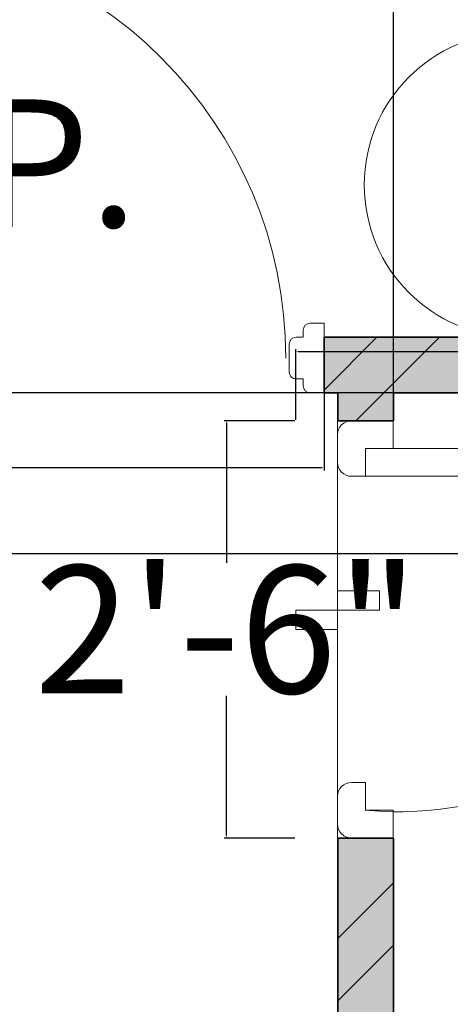
# Model space of a CAD drawing. Units: inches. Extents: x 1086 to 1540, y 3343 to 3848.
# Tile 4 of 8: x 1350 to 1381, y 3591 to 3661. Entities that reach past the tile are written whole.
import ezdxf

# ---------------------------------------------------------------- set-up
doc = ezdxf.new("R2010")
doc.units = ezdxf.units.IN
for name, color, linetype, lineweight in [('00 FURNITURE', 15, 'Continuous', 15), ('A-ANNO-DIMS', 2, 'Continuous', 13), ('A-DOOR', 4, 'Continuous', 20), ('A-WALL-PATT', 252, 'Continuous', 9), ('A_FUR 1', 5, 'Continuous', 5), ('WALL', 7, 'Continuous', 35)]:
    doc.layers.add(name, color=color, linetype=linetype, lineweight=lineweight)
doc.styles.get("Standard").update_dxf_attribs({"font": 'arial.ttf'})
doc.dimstyles.get("Standard").update_dxf_attribs({"dimtxt": 9.18, "dimasz": 0.18, "dimexe": 0.18, "dimexo": 0.0625, "dimgap": 0.09, "dimtad": 0, "dimtih": 1, "dimtoh": 1, "dimdec": 1, "dimzin": 0, "dimdsep": 46, "dimlunit": 3, "dimtxsty": 'Standard', "dimcen": 0.09, "dimadec": 0, "dimazin": 0, "dimtfac": 1, "dimtdec": 1, "dimtofl": 0, "dimtmove": 0, "dimatfit": 3, "dimfxl": 1, "dimtolj": 1, "dimtzin": 0, "dimarcsym": 0})

# ---------------------------------------------------------------- blocks, each defined once
blk = doc.blocks.new('DDD')
at = {"layer": '00 FURNITURE'}
for p, q in [((-12579.77346126611, -15859.52901419652), (-12579.77346126608, -15829.04541204713)), ((-12578.77346126611, -15859.52901419657), (-12578.77346126608, -15829.02901419657)), ((-12612.02346126613, -15857.02901419646), (-12612.02346126613, -15862.02901419646)), ((-12611.02346126613, -15857.02901419646), (-12612.02346126613, -15857.02901419646)), ((-12610.52346126612, -15858.02901419646), (-12610.52346126612, -15857.52901419646)), ((-12577.52346126611, -15858.02901419658), (-12577.52346126611, -15857.52901419657)), ((-12577.02346126611, -15857.02901419657), (-12576.02346126611, -15857.02901419652)), ((-12576.02346126611, -15857.02901419652), (-12576.02346126611, -15862.02901419652)), ((-12578.77346126611, -15859.52901419657), (-12579.77346126611, -15859.52901419652)), ((-12610.52346126612, -15861.52901419646), (-12610.52346126612, -15861.02901419646)), ((-12577.52346126611, -15861.52901419657), (-12577.52346126611, -15861.02901419657)), ((-12612.02346126613, -15862.02901419646), (-12611.02346126613, -15862.02901419646)), ((-12576.02346126611, -15862.02901419652), (-12577.02346126611, -15862.02901419657))]:
    blk.add_line(p, q, dxfattribs=at)
for points in [[(-12610.52346126612, -15861.02901419646), (-12610.02346126613, -15861.02901419646, 0.4142135623730951), (-12609.52346126612, -15860.52901419646), (-12609.52346126612, -15858.52901419646, 0.4142135623730951), (-12610.02346126613, -15858.02901419646), (-12610.52346126612, -15858.02901419646)], [(-12577.52346126611, -15861.02901419657), (-12578.02346126611, -15861.02901419657, -0.4142135623730951), (-12578.52346126611, -15860.52901419657), (-12578.52346126611, -15858.52901419657, -0.4142135623730951), (-12578.02346126611, -15858.02901419658), (-12577.52346126611, -15858.02901419658)]]:
    blk.add_lwpolyline(points, format="xyb", dxfattribs=at)
for centre, radius, start, end in [((-12578.77346126613, -15859.52901419657), 30.49999999999949, 90, 180), ((-12611.02346126613, -15857.52901419646), 0.4999999999999916, 0, 90), ((-12577.02346126611, -15857.52901419657), 0.4999999999999916, 90, 180), ((-12611.02346126613, -15861.52901419646), 0.4999999999999916, 270, 0), ((-12577.02346126611, -15861.52901419657), 0.4999999999999916, 180, 270)]:
    blk.add_arc(centre, radius, start, end, dxfattribs=at)
blk = doc.blocks.new('ESTSET')
at = {"layer": 'A_FUR 1'}
for p, q in [((-10.44359699611232, 4.096573562603225), (-10.44359699611232, 32.09657356260323)), ((-8.44359699611232, 4.096573562603225), (-8.44359699611232, 32.09657356260323)), ((-36.44359699611232, 6.096573562603225), (-36.44359699611232, 3.096573562603225)), ((-34.44359699611232, 6.096573562603225), (-36.44359699611232, 6.096573562603225)), ((-34.44359699611232, 4.096573562603225), (-34.44359699611232, 6.096573562603225)), ((-34.44359699611232, 4.096573562603225), (-34.44359699611232, 6.096573562603225)), ((-8.44359699611232, 4.096573562603225), (-8.44359699611232, 6.096573562603225)), ((-8.44359699611232, 6.096573562603225), (-6.443596996112319, 6.096573562603225)), ((-8.44359699611232, 4.096573562603225), (-8.44359699611232, 6.096573562603225)), ((-6.443596996112319, 6.096573562603225), (-6.443596996112319, 3.096573562603225)), ((-32.44359699611232, 4.096573562603225), (-34.44359699611232, 4.096573562603225)), ((-32.44359699611232, 4.096573562603225), (-34.44359699611232, 4.096573562603225)), ((-32.44359699611232, 3.096573562603225), (-32.44359699611232, 4.096573562603225)), ((-10.44359699611232, 3.096573562603225), (-10.44359699611232, 4.096573562603225)), ((-10.44359699611232, 4.096573562603225), (-8.44359699611232, 4.096573562603225)), ((-10.44359699611232, 4.096573562603225), (-8.44359699611232, 4.096573562603225)), ((-6.443596996112319, 2.096573562601521), (-36.4435969961196, 2.09657356260334)), ((-35.44359699611232, 2.096573562603225), (-33.44359699611232, 2.096573562603225)), ((-7.443596996112319, 2.096573562603225), (-9.44359699611232, 2.096573562603225))]:
    blk.add_line(p, q, dxfattribs=at)
for points in [[(-21.44359699614506, 2.09657356260334), (-18.67227073841423, 2.09657356260334), (-18.67227073841423, 5.101808480258228), (-20.05793386727964, 5.101808480258228)], [(-20.05793386727964, 5.101808480258228), (-20.05793386727964, -0.9086613550515485)], [(-21.44359699614506, 2.09657356260334), (-21.44359699614506, -0.9086613550515485), (-20.05793386727964, -0.9086613550515485)]]:
    blk.add_lwpolyline(points, dxfattribs=at)
for centre, radius, start, end in [((-8.908777800232201, 6.457098594999479), 25.64369454261379, 88.96058819788949, 185.2816045955121), ((-35.44359699611232, 3.096573562603225), 1, 180, 270), ((-33.44359699611232, 3.096573562603225), 1, 270, 0), ((-9.44359699611232, 3.096573562603225), 1, 180, 270), ((-7.443596996112319, 3.096573562603225), 1, 270, 0)]:
    blk.add_arc(centre, radius, start, end, dxfattribs=at)
blk = doc.blocks.new('TABLE-ROUND-SIDE')
blk.add_circle((2.274e-13, 0), 10.94980314960581)
blk = doc.blocks.new('*D25')
at = {"layer": 'A-ANNO-DIMS', "color": 0, "lineweight": -2, "transparency": 16777216}
for p, q in [((1335.7404436631, 3634.50827962207), (1335.7404436631, 3628.990779622068)), ((1371.74044366312, 3634.50827962207), (1371.74044366312, 3628.990779622068)), ((1335.7404436631, 3629.170779622067), (1335.5604436631, 3629.170779622067)), ((1371.56044366312, 3629.170779622067), (1335.9204436631, 3629.170779622067))]:
    blk.add_line(p, q, dxfattribs=at)
at = {"layer": 'A-ANNO-DIMS', "color": 0, "transparency": 16777216}
for points in [[(1335.9204436631, 3629.200779622067), (1335.9204436631, 3629.140779622067), (1335.7404436631, 3629.170779622067)], [(1371.56044366312, 3629.200779622067), (1371.56044366312, 3629.140779622067), (1371.74044366312, 3629.170779622067)]]:
    blk.add_solid(points, dxfattribs=at)
at = {"layer": 'Defpoints', "color": 0, "transparency": 16777216}
for p in [(1335.7404436631, 3634.570779622071), (1371.74044366312, 3634.570779622071), (1335.7404436631, 3629.170779622067)]:
    blk.add_point(p, dxfattribs=at)
at = {"layer": 'A-ANNO-DIMS', "color": 0, "transparency": 16777216, "insert": (1251.763997551231, 3629.170779622067), "char_height": 9.18, "attachment_point": 5}
blk.add_mtext('\\A1;BEDROOM DOOR 3\'-0" TYP.', dxfattribs=at)
blk = doc.blocks.new('*D26')
at = {"layer": 'A-ANNO-DIMS', "color": 0, "lineweight": -2, "transparency": 16777216}
for p, q in [((1335.677943663101, 3667.570779622072), (1330.160443663098, 3667.570779622072)), ((1330.340443663098, 3667.390779622073), (1330.340443663098, 3655.847839649358)), ((1330.340443663098, 3634.750779622072), (1330.340443663098, 3646.293719594787)), ((1335.677943663101, 3634.570779622072), (1330.160443663098, 3634.570779622072))]:
    blk.add_line(p, q, dxfattribs=at)
at = {"layer": 'A-ANNO-DIMS', "color": 0, "transparency": 16777216}
for points in [[(1330.310443663098, 3667.390779622073), (1330.370443663098, 3667.390779622073), (1330.340443663098, 3667.570779622072)], [(1330.310443663098, 3634.750779622072), (1330.370443663098, 3634.750779622072), (1330.340443663098, 3634.570779622072)]]:
    blk.add_solid(points, dxfattribs=at)
at = {"layer": 'Defpoints', "color": 0, "transparency": 16777216}
for p in [(1330.340443663098, 3667.570779622072), (1335.740443663101, 3667.570779622072), (1335.740443663101, 3634.570779622072)]:
    blk.add_point(p, dxfattribs=at)
at = {"layer": 'A-ANNO-DIMS', "color": 0, "transparency": 16777216, "insert": (1330.340443663099, 3651.070779622071), "char_height": 9.18, "attachment_point": 5}
blk.add_mtext('\\A1;2\'-9" TYP.', dxfattribs=at)
blk = doc.blocks.new('*D41')
at = {"layer": 'A-ANNO-DIMS', "color": 0, "lineweight": -2, "transparency": 16777216}
for p, q in [((1369.709395983253, 3632.633280204329), (1369.709395983253, 3637.721409000223)), ((1402.846921289218, 3632.633280204329), (1402.846921289218, 3637.721409000223)), ((1369.889395983253, 3637.541409000223), (1402.666921289218, 3637.541409000223)), ((1402.846921289218, 3637.541409000223), (1403.026921289218, 3637.541409000223))]:
    blk.add_line(p, q, dxfattribs=at)
at = {"layer": 'A-ANNO-DIMS', "color": 0, "transparency": 16777216}
for points in [[(1369.889395983253, 3637.571409000223), (1369.889395983253, 3637.511409000223), (1369.709395983253, 3637.541409000223)], [(1402.666921289218, 3637.571409000223), (1402.666921289218, 3637.511409000223), (1402.846921289218, 3637.541409000223)]]:
    blk.add_solid(points, dxfattribs=at)
at = {"layer": 'Defpoints', "color": 0, "transparency": 16777216}
for p in [(1402.846921289218, 3637.541409000223), (1369.709395983253, 3632.570780204329), (1402.846921289218, 3632.570780204329)]:
    blk.add_point(p, dxfattribs=at)
at = {"layer": 'A-ANNO-DIMS', "color": 0, "transparency": 16777216, "insert": (1460.679779406544, 3637.541409000223), "char_height": 9.18, "attachment_point": 5}
blk.add_mtext('\\A1;TOILET DOOR 2\'-9"', dxfattribs=at)
blk = doc.blocks.new('*D42')
at = {"layer": 'A-ANNO-DIMS', "color": 0, "lineweight": -2, "transparency": 16777216}
for p, q in [((1369.646895983254, 3632.570780204331), (1364.558767187359, 3632.570780204331)), ((1364.73876718736, 3632.390780204331), (1364.73876718736, 3622.347840231612)), ((1364.73876718736, 3602.750780204323), (1364.73876718736, 3612.793720177041)), ((1369.646895983254, 3602.570780204323), (1364.558767187359, 3602.570780204323))]:
    blk.add_line(p, q, dxfattribs=at)
at = {"layer": 'A-ANNO-DIMS', "color": 0, "transparency": 16777216}
for points in [[(1364.708767187359, 3632.390780204331), (1364.768767187359, 3632.390780204331), (1364.73876718736, 3632.570780204331)], [(1364.708767187359, 3602.750780204323), (1364.768767187359, 3602.750780204323), (1364.73876718736, 3602.570780204323)]]:
    blk.add_solid(points, dxfattribs=at)
at = {"layer": 'Defpoints', "color": 0, "transparency": 16777216}
for p in [(1364.73876718736, 3632.570780204331), (1369.709395983254, 3632.570780204331), (1369.709395983254, 3602.570780204323)]:
    blk.add_point(p, dxfattribs=at)
at = {"layer": 'A-ANNO-DIMS', "color": 0, "transparency": 16777216, "insert": (1364.73876718736, 3617.570780204326), "char_height": 9.18, "attachment_point": 5}
blk.add_mtext('\\A1;2\'-6"', dxfattribs=at)
blk = doc.blocks.new('*D69')
at = {"layer": 'A-ANNO-DIMS', "color": 0, "lineweight": -2, "transparency": 16777216}
for p, q in [((1421.677948, 3634.570780000002), (1171.560448000001, 3634.570780000002)), ((1171.740448000001, 3634.390780000002), (1171.740448000001, 3633.620340431107)), ((1171.740448000001, 3623.176804000002), (1171.740448000001, 3623.947243568897)), ((1420.43861, 3622.996804000002), (1171.560448000001, 3622.996804000002))]:
    blk.add_line(p, q, dxfattribs=at)
at = {"layer": 'A-ANNO-DIMS', "color": 0, "transparency": 16777216}
for points in [[(1171.710448000001, 3634.390780000002), (1171.770448000001, 3634.390780000002), (1171.740448000001, 3634.570780000002)], [(1171.710448000001, 3623.176804000002), (1171.770448000001, 3623.176804000002), (1171.740448000001, 3622.996804000002)]]:
    blk.add_solid(points, dxfattribs=at)
at = {"layer": 'Defpoints', "color": 0, "transparency": 16777216}
for p in [(1421.740448, 3634.570780000002), (1171.740448000001, 3622.996804000002), (1420.50111, 3622.996804000002)]:
    blk.add_point(p, dxfattribs=at)
at = {"layer": 'A-ANNO-DIMS', "color": 0, "transparency": 16777216, "insert": (1171.740448000002, 3628.783792), "char_height": 9.18, "attachment_point": 5}
blk.add_mtext('\\A1;0\'-11 1/2"', dxfattribs=at)
blk = doc.blocks.new('*D70')
at = {"layer": 'A-ANNO-DIMS', "color": 0, "lineweight": -2, "transparency": 16777216}
for p, q in [((1376.740448, 3634.63328), (1376.740448, 3834.75078)), ((1376.920448, 3834.57078), (1386.952194248294, 3834.57078)), ((1421.560448, 3834.57078), (1411.528701751705, 3834.57078)), ((1421.740448, 3634.63328), (1421.740448, 3834.75078))]:
    blk.add_line(p, q, dxfattribs=at)
at = {"layer": 'A-ANNO-DIMS', "color": 0, "transparency": 16777216}
for points in [[(1376.920448, 3834.60078), (1376.920448, 3834.54078), (1376.740448, 3834.57078)], [(1421.560448, 3834.60078), (1421.560448, 3834.54078), (1421.740448, 3834.57078)]]:
    blk.add_solid(points, dxfattribs=at)
at = {"layer": 'Defpoints', "color": 0, "transparency": 16777216}
for p in [(1421.740448, 3834.57078), (1376.740448, 3634.57078), (1421.740448, 3634.57078)]:
    blk.add_point(p, dxfattribs=at)
at = {"layer": 'A-ANNO-DIMS', "color": 0, "transparency": 16777216, "insert": (1399.240448, 3834.57078), "char_height": 9.18, "attachment_point": 5}
blk.add_mtext('\\A1;3\'-9"', dxfattribs=at)

msp = doc.modelspace()

# ---------------------------------------------------------------- hatches: boundary and pattern name
at = {"layer": 'A-WALL-PATT'}
h = msp.add_hatch(dxfattribs=at)
h.set_pattern_fill('ANSI32', color=256)
h.set_pattern_definition([(45, (0, 0), (-6.735192090801865, 6.735192090801866), []), (45, (4.49013, 0), (-6.735192090801865, 6.735192090801866), [])])
h.paths.add_polyline_path([(1234.550507268797, 3811.570780184086), (1234.550506085547, 3811.570780184086), (1194.74044790643, 3811.570780204329), (1194.74044790643, 3622.570780204329), (1203.74044790643, 3622.570780204329), (1203.74044790643, 3634.57078020433), (1218.334481095046, 3634.57078020433), (1218.334481095046, 3638.570780204329), (1203.74044790643, 3638.570780204329), (1203.74044790643, 3802.570780204329), (1234.550507268797, 3802.570780204328)])
h.paths.add_polyline_path([(1371.059017457095, 3811.570780184086), (1371.059016273845, 3811.570780184086), (1282.550507268797, 3811.570780204329), (1282.550507268797, 3802.570780204328), (1331.74044790643, 3802.570780204329), (1331.74044790643, 3634.57078020433), (1335.740443663098, 3634.570780204329), (1335.740443663098, 3639.570779622127), (1335.74044790643, 3802.570780204329), (1371.059017457095, 3802.570780204329)])
h.paths.add_polyline_path([(1470.74044790643, 3811.570780204329), (1419.059017457095, 3811.570780204329), (1419.059017457094, 3802.570780204329), (1461.74044790643, 3802.570780204329), (1461.74044790643, 3638.570780204329), (1461.74044790643, 3548.570780204335), (1425.74044790643, 3548.570780204334), (1425.74044790643, 3582.213777424251), (1421.74044790643, 3582.213777424251), (1421.74044790643, 3548.570780204334), (1376.74044790643, 3548.570780204333), (1376.74044790643, 3602.570780204329), (1373.714630900908, 3602.570780204329), (1372.74044790643, 3602.570780204329), (1372.74044790643, 3544.570780204329), (1461.74044790643, 3544.570780204332), (1461.74044790643, 3379.57078020433), (1470.74044790643, 3379.570780204329)])
h.paths.add_polyline_path([(1203.74044790643, 3582.570780204329), (1295.74044790643, 3582.57078020433), (1295.74044790643, 3586.57078020433), (1203.74044790643, 3586.570780204329), (1203.74044790643, 3598.570780204329), (1194.74044790643, 3598.570780204329), (1194.74044790643, 3379.570780204329), (1326.74044790643, 3379.570780204329), (1326.74044790643, 3388.570780204329), (1322.74044790643, 3388.570780204329), (1203.74044790643, 3388.570780204329), (1203.74044790643, 3451.570780204329), (1234.74044790643, 3451.570780204329), (1234.740447906429, 3455.570780204329), (1203.74044790643, 3455.570780204329), (1203.74044790643, 3479.570780204329), (1203.74044790643, 3544.570780204329), (1227.74044790643, 3544.570780204329), (1253.74044790643, 3544.570780204329), (1253.74044790643, 3548.570780204329), (1203.74044790643, 3548.570780204329)])
h.paths.add_polyline_path([(1461.74044790643, 3638.570780204329), (1371.74044790643, 3638.570780204329), (1371.74044790643, 3634.570780204329), (1372.74044790643, 3634.57078020433), (1372.74044790643, 3632.570780204328), (1376.74044790643, 3632.570780204328), (1376.74044790643, 3634.570780204329), (1421.74044790643, 3634.57078020433), (1421.74044790643, 3606.21377742425), (1425.74044790643, 3606.213777424251), (1425.74044790643, 3634.57078020433), (1461.74044790643, 3634.57078020433)])
h.paths.add_polyline_path([(1295.740445944246, 3638.570780204329), (1266.334481095045, 3638.570780204329), (1266.334481095045, 3634.57078020433), (1292.74044790643, 3634.57078020433), (1295.740445944246, 3634.57078020433)])
h.paths.add_polyline_path([(1322.74044790643, 3548.570780204332), (1318.74044790643, 3548.570780204331), (1318.74044790643, 3455.570780204329), (1282.74044790643, 3455.570780204329), (1282.74044790643, 3451.57078020433), (1318.74044790643, 3451.57078020433), (1318.74044790643, 3420.07078020433), (1322.74044790643, 3420.07078020433)], flags=17)
at = {"layer": 'A-WALL-PATT', "transparency": 33554559}
h = msp.add_hatch(color=256, dxfattribs=at)
h.dxf.hatch_style = 1
h.paths.add_polyline_path([(1234.550507268797, 3811.570780184086), (1234.550506085547, 3811.570780184086), (1194.74044790643, 3811.570780204329), (1194.74044790643, 3622.570780204329), (1203.74044790643, 3622.570780204329), (1203.74044790643, 3634.57078020433), (1218.334481095046, 3634.57078020433), (1218.334481095046, 3638.570780204329), (1203.74044790643, 3638.570780204329), (1203.74044790643, 3802.570780204329), (1234.550507268797, 3802.570780204328)])
h.paths.add_polyline_path([(1371.059017457095, 3811.570780184086), (1371.059016273845, 3811.570780184086), (1282.550507268797, 3811.570780204329), (1282.550507268797, 3802.570780204328), (1331.74044790643, 3802.570780204329), (1331.74044790643, 3634.57078020433), (1335.740443663098, 3634.570780204329), (1335.740443663098, 3639.570779622127), (1335.74044790643, 3802.570780204329), (1371.059017457095, 3802.570780204329)])
h.paths.add_polyline_path([(1470.74044790643, 3811.570780204329), (1419.059017457095, 3811.570780204329), (1419.059017457094, 3802.570780204329), (1461.74044790643, 3802.570780204329), (1461.74044790643, 3638.570780204329), (1461.74044790643, 3548.570780204335), (1425.74044790643, 3548.570780204334), (1425.74044790643, 3582.213777424251), (1421.74044790643, 3582.213777424251), (1421.74044790643, 3548.570780204334), (1376.74044790643, 3548.570780204333), (1376.74044790643, 3602.570780204328), (1372.74044790643, 3602.570780204329), (1372.74044790643, 3544.570780204329), (1461.74044790643, 3544.570780204332), (1461.74044790643, 3379.57078020433), (1470.74044790643, 3379.570780204329)])
h.paths.add_polyline_path([(1203.74044790643, 3544.570780204329), (1227.74044790643, 3544.570780204329), (1253.74044790643, 3544.570780204329), (1253.74044790643, 3548.570780204329), (1203.74044790643, 3548.570780204329), (1203.74044790643, 3582.570780204329), (1295.74044790643, 3582.57078020433), (1295.74044790643, 3586.57078020433), (1203.74044790643, 3586.570780204329), (1203.74044790643, 3598.570780204329), (1194.74044790643, 3598.570780204329), (1194.74044790643, 3379.570780204329), (1326.74044790643, 3379.570780204329), (1326.74044790643, 3388.570780204329), (1322.74044790643, 3388.570780204329), (1203.74044790643, 3388.570780204329), (1203.74044790643, 3451.570780204329), (1234.74044790643, 3451.570780204329), (1234.740447906429, 3455.570780204329), (1203.74044790643, 3455.570780204329)])
h.paths.add_polyline_path([(1413.74044790643, 3388.570780184088), (1413.740446723181, 3388.570780184088), (1374.74044790643, 3388.570780204329), (1374.74044790643, 3383.179800700248), (1374.74045402255, 3383.179800700248), (1374.740454022761, 3379.570780204329), (1413.74044790643, 3379.57078020433)], flags=17)
h.paths.add_polyline_path([(1322.74044790643, 3548.570780204332), (1318.74044790643, 3548.570780204331), (1318.74044790643, 3455.570780204329), (1282.74044790643, 3455.570780204329), (1282.74044790643, 3451.57078020433), (1318.74044790643, 3451.57078020433), (1318.74044790643, 3420.07078020433), (1322.74044790643, 3420.07078020433)], flags=17)
h.paths.add_polyline_path([(1295.740445944246, 3638.570780204329), (1266.334481095045, 3638.570780204329), (1266.334481095045, 3634.57078020433), (1292.74044790643, 3634.57078020433), (1295.740445944246, 3634.57078020433)])
h.paths.add_polyline_path([(1461.74044790643, 3638.570780204329), (1371.74044790643, 3638.570780204329), (1371.74044790643, 3634.570780204329), (1372.74044790643, 3634.57078020433), (1372.74044790643, 3632.570780204328), (1376.74044790643, 3632.570780204328), (1376.74044790643, 3634.570780204329), (1421.74044790643, 3634.57078020433), (1421.74044790643, 3606.21377742425), (1425.74044790643, 3606.213777424251), (1425.74044790643, 3634.57078020433), (1461.74044790643, 3634.57078020433)])

# ---------------------------------------------------------------- linework, layer by layer
at = {"layer": 'WALL'}
for p, q in [((1371.74044790643, 3638.570780204329), (1461.74044790643, 3638.570780204329)), ((1371.74044790643, 3634.570780204328), (1371.74044790643, 3638.570780204328)), ((1371.74044790643, 3634.570780204329), (1372.74044790643, 3634.57078020433)), ((1372.74044790643, 3634.570780204329), (1372.74044790643, 3632.570780204328)), ((1376.74044790643, 3634.570780204329), (1376.74044790643, 3632.570780204328)), ((1376.74044790643, 3634.570780204329), (1421.74044790643, 3634.57078020433)), ((1372.74044790643, 3632.570780204328), (1376.74044790643, 3632.570780204328)), ((1372.74044790643, 3602.570780204329), (1376.74044790643, 3602.570780204328)), ((1372.74044790643, 3602.570780204329), (1372.74044790643, 3544.57078020433)), ((1376.74044790643, 3602.57078020433), (1376.74044790643, 3548.570780204333))]:
    msp.add_line(p, q, dxfattribs=at)

# ---------------------------------------------------------------- block references
at = {"layer": '00 FURNITURE'}
msp.add_blockref('TABLE-ROUND-SIDE', (1385.585271056955, 3649.520582927621), dxfattribs=at)
at = {"layer": 'A-DOOR', "xscale": -1}
msp.add_blockref('DDD', (-11240.28301760301, 19496.59979381864), dxfattribs=at)
at = {"layer": 'A-DOOR', "xscale": -1, "rotation": 270}
msp.add_blockref('ESTSET', (1370.618057338305, 3639.014377200441), dxfattribs=at)

# ---------------------------------------------------------------- dimensions: what is measured, and where the dimension line sits
at = {"layer": 'A-ANNO-DIMS'}
dim = msp.add_linear_dim(base=(1421.740448, 3834.57078), p1=(1376.740448, 3634.57078), p2=(1421.740448, 3634.57078), dimstyle='Standard', override={"dimdec": 1, "dimlfac": 1, "dimrnd": 0, "dimzin": 1, "dimdsep": 46, "dimlunit": 4, "dimfrac": 2}, dxfattribs=at)
dim.commit()
dim.dimension.update_dxf_attribs({"geometry": '*D70', "text_midpoint": (1399.240448, 3834.57078)})
for base, p1, p2, angle, text, picture, middle in [((1330.340443663098, 3667.570779622072), (1335.7404436631, 3634.570779622071), (1335.7404436631, 3667.570779622071), 90, '<> TYP.', '*D26', (1330.340443663099, 3651.070779622071)), ((1335.7404436631, 3629.170779622067), (1371.74044366312, 3634.570779622071), (1335.7404436631, 3634.570779622071), 180, 'BEDROOM DOOR <> TYP.', '*D25', (1251.763997551231, 3629.170779622067))]:
    dim = msp.add_linear_dim(base=base, p1=p1, p2=p2, angle=angle, text=text, dimstyle='Standard', override={"dimdec": 1, "dimlfac": 1, "dimrnd": 0, "dimzin": 1, "dimdsep": 46, "dimlunit": 4, "dimfrac": 2}, dxfattribs=at)
    dim.commit()
    dim.dimension.update_dxf_attribs({"geometry": picture, "text_midpoint": middle})
dim = msp.add_linear_dim(base=(1402.846921289218, 3637.541409000223), p1=(1369.709395983253, 3632.570780204329), p2=(1402.846921289218, 3632.570780204329), text='TOILET DOOR <>', dimstyle='Standard', override={"dimdec": 1, "dimlfac": 1, "dimrnd": 0, "dimzin": 1, "dimdsep": 46, "dimlunit": 4, "dimfrac": 2}, dxfattribs=at)
dim.commit()
dim.dimension.update_dxf_attribs({"geometry": '*D41', "text_midpoint": (1460.679779406544, 3637.541409000223)})
for base, p1, p2, picture, middle in [((1171.740448000001, 3622.996804000002), (1421.740448, 3634.57078), (1420.50111, 3622.996804), '*D69', (1171.740448000002, 3628.783792)), ((1364.73876718736, 3632.570780204331), (1369.709395983253, 3602.570780204322), (1369.709395983253, 3632.570780204329), '*D42', (1364.73876718736, 3617.570780204326))]:
    dim = msp.add_linear_dim(base=base, p1=p1, p2=p2, angle=90, dimstyle='Standard', override={"dimdec": 1, "dimlfac": 1, "dimrnd": 0, "dimzin": 1, "dimdsep": 46, "dimlunit": 4, "dimfrac": 2}, dxfattribs=at)
    dim.commit()
    dim.dimension.update_dxf_attribs({"geometry": picture, "text_midpoint": middle})

doc.saveas('drawing.dxf')
